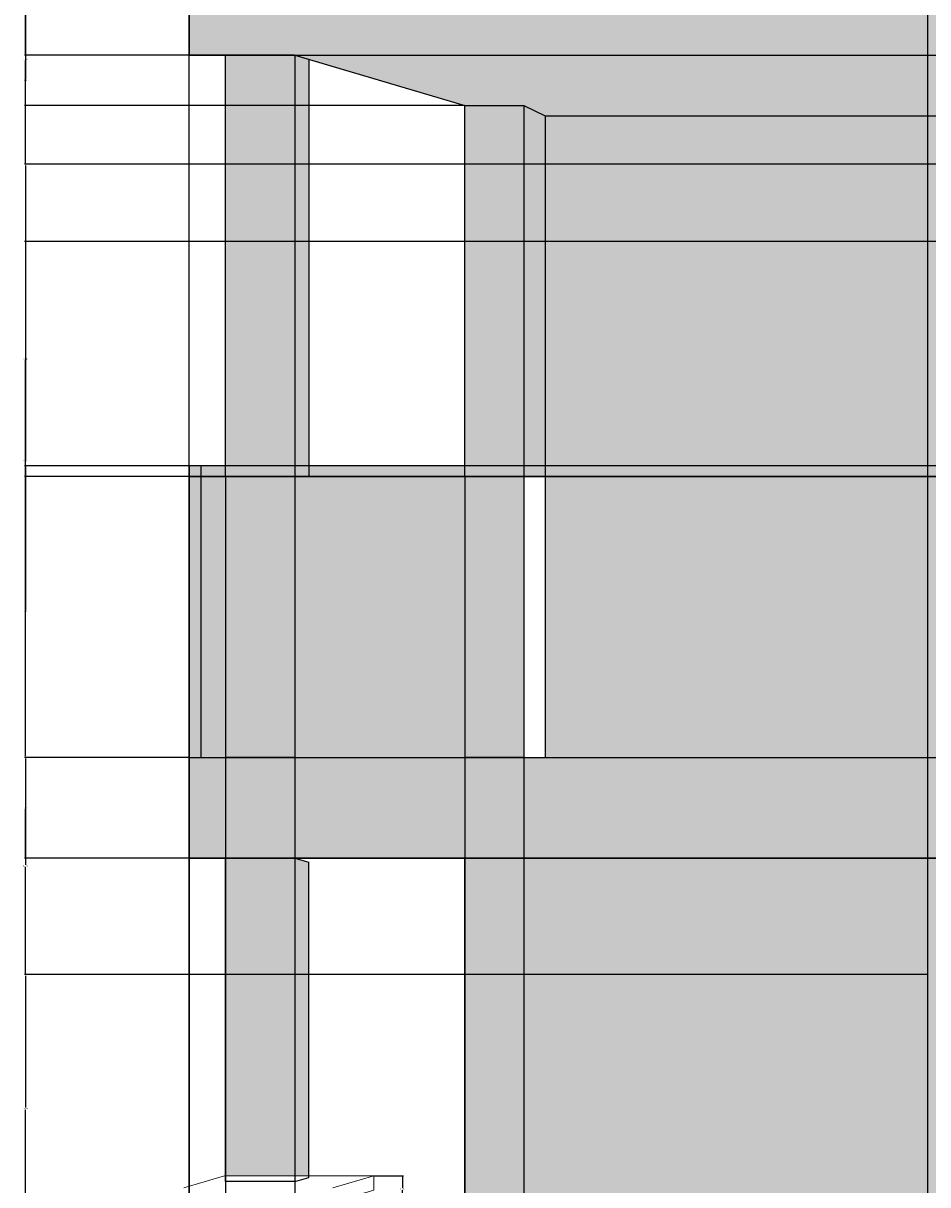
# Model space of a CAD drawing. Units: feet. Extents: x 2926 to 4178, y 965 to 1469.
# Tile 2 of 9: x 2926 to 3068, y 1059 to 1241. Entities that reach past the tile are written whole.
import ezdxf

# ---------------------------------------------------------------- set-up
doc = ezdxf.new("R2010")
doc.units = ezdxf.units.FT
for name, color, linetype, lineweight in [('A-ANNO-DIMS', 2, 'Continuous', 18), ('A-ELEV', 7, 'Continuous', 25), ('A-ELEV-DETL', 8, 'Continuous', 18), ('A-ELEV-PATT', 9, 'Continuous', 13)]:
    doc.layers.add(name, color=color, linetype=linetype, lineweight=lineweight)
doc.styles.get("Standard").update_dxf_attribs({"font": 'arial.ttf'})
doc.dimstyles.get("Standard").update_dxf_attribs({"dimtxt": 0.18, "dimasz": 0.18, "dimexe": 0.18, "dimexo": 0.0625, "dimgap": 0.09, "dimtad": 0, "dimtih": 1, "dimtoh": 1, "dimdec": 1, "dimzin": 0, "dimdsep": 46, "dimlunit": 3, "dimtxsty": 'Standard', "dimcen": 0.09, "dimadec": 0, "dimazin": 0, "dimtfac": 1, "dimtdec": 1, "dimtofl": 0, "dimtmove": 0, "dimatfit": 3, "dimfxl": 1, "dimtolj": 1, "dimtzin": 0, "dimarcsym": 0})

# ---------------------------------------------------------------- blocks, each defined once
blk = doc.blocks.new('PILLAR-CAP-A')
for p, q in [((0, 2.25), (6.42, 4.14)), ((0, 2.25), (6.42, 4.14)), ((29.85, 4.14), (6.42, 4.14)), ((29.85, 4.14), (6.42, 4.14)), ((23.43, 2.25), (29.85, 4.14)), ((23.43, 2.25), (29.85, 4.14)), ((29.85, 1.89), (29.85, 4.14)), ((29.85, 1.89), (29.85, 4.14)), ((23.43, 0), (29.85, 1.89)), ((23.43, 0), (29.85, 1.89))]:
    blk.add_line(p, q)
blk = doc.blocks.new('*D7')
at = {"layer": 'A-ANNO-DIMS', "color": 0, "lineweight": -2, "transparency": 16777216}
for p, q in [((2981.46, 1060.46), (2986.06, 1060.46)), ((2985.88, 1060.28), (2985.88, 1058.57)), ((2985.88, 1056.5), (2985.88, 1058.21)), ((2981.46, 1056.32), (2986.06, 1056.32))]:
    blk.add_line(p, q, dxfattribs=at)
at = {"layer": 'A-ANNO-DIMS', "color": 0, "transparency": 16777216}
for points in [[(2985.85, 1060.28), (2985.91, 1060.28), (2985.88, 1060.46)], [(2985.85, 1056.5), (2985.91, 1056.5), (2985.88, 1056.32)]]:
    blk.add_solid(points, dxfattribs=at)
at = {"layer": 'Defpoints', "color": 0, "transparency": 16777216}
for p in [(2981.4, 1060.46), (2985.88, 1060.46), (2981.4, 1056.32)]:
    blk.add_point(p, dxfattribs=at)
at = {"layer": 'A-ANNO-DIMS', "color": 0, "transparency": 16777216, "insert": (2985.88, 1058.39), "char_height": 0.18, "attachment_point": 5}
blk.add_mtext('\\A1;4 TYP.', dxfattribs=at)
blk = doc.blocks.new('*D14')
at = {"layer": 'A-ANNO-DIMS', "color": 0, "lineweight": -2, "transparency": 16777216}
for p, q in [((3068.25, 1092.04), (2926.57, 1092.04)), ((2926.75, 1091.86), (2926.75, 1071.2)), ((2926.75, 1050.16), (2926.75, 1070.83)), ((3068.25, 1049.98), (2926.57, 1049.98))]:
    blk.add_line(p, q, dxfattribs=at)
at = {"layer": 'A-ANNO-DIMS', "color": 0, "transparency": 16777216}
for points in [[(2926.72, 1091.86), (2926.78, 1091.86), (2926.75, 1092.04)], [(2926.72, 1050.16), (2926.78, 1050.16), (2926.75, 1049.98)]]:
    blk.add_solid(points, dxfattribs=at)
at = {"layer": 'Defpoints', "color": 0, "transparency": 16777216}
for p in [(2926.75, 1092.04), (3068.31, 1092.04), (3068.31, 1049.98)]:
    blk.add_point(p, dxfattribs=at)
at = {"layer": 'A-ANNO-DIMS', "color": 0, "transparency": 16777216, "insert": (2926.75, 1071.01), "char_height": 0.18, "attachment_point": 5}
blk.add_mtext('\\A1;42.06', dxfattribs=at)
blk = doc.blocks.new('*D15')
at = {"layer": 'A-ANNO-DIMS', "color": 0, "lineweight": -2, "transparency": 16777216}
for p, q in [((2952.34, 1126.14), (2926.57, 1126.14)), ((2926.75, 1125.96), (2926.75, 1109.27)), ((2926.75, 1092.22), (2926.75, 1108.91)), ((3068.25, 1092.04), (2926.57, 1092.04))]:
    blk.add_line(p, q, dxfattribs=at)
at = {"layer": 'A-ANNO-DIMS', "color": 0, "transparency": 16777216}
for points in [[(2926.72, 1125.96), (2926.78, 1125.96), (2926.75, 1126.14)], [(2926.72, 1092.22), (2926.78, 1092.22), (2926.75, 1092.04)]]:
    blk.add_solid(points, dxfattribs=at)
at = {"layer": 'Defpoints', "color": 0, "transparency": 16777216}
for p in [(2926.75, 1126.14), (2952.4, 1126.14), (3068.31, 1092.04)]:
    blk.add_point(p, dxfattribs=at)
at = {"layer": 'A-ANNO-DIMS', "color": 0, "transparency": 16777216, "insert": (2926.75, 1109.09), "char_height": 0.18, "attachment_point": 5}
blk.add_mtext('\\A1;34.095', dxfattribs=at)
blk = doc.blocks.new('*D16')
at = {"layer": 'A-ANNO-DIMS', "color": 0, "lineweight": -2, "transparency": 16777216}
for p, q in [((3198.58, 1219.22), (2926.57, 1219.22)), ((2926.75, 1219.04), (2926.75, 1172.86)), ((2926.75, 1126.32), (2926.75, 1172.5)), ((2952.34, 1126.14), (2926.57, 1126.14))]:
    blk.add_line(p, q, dxfattribs=at)
at = {"layer": 'A-ANNO-DIMS', "color": 0, "transparency": 16777216}
for points in [[(2926.72, 1219.04), (2926.78, 1219.04), (2926.75, 1219.22)], [(2926.72, 1126.32), (2926.78, 1126.32), (2926.75, 1126.14)]]:
    blk.add_solid(points, dxfattribs=at)
at = {"layer": 'Defpoints', "color": 0, "transparency": 16777216}
for p in [(2926.75, 1219.22), (3198.64, 1219.22), (2952.4, 1126.14)]:
    blk.add_point(p, dxfattribs=at)
at = {"layer": 'A-ANNO-DIMS', "color": 0, "transparency": 16777216, "insert": (2926.75, 1172.68), "char_height": 0.18, "attachment_point": 5}
blk.add_mtext('\\A1;93.08', dxfattribs=at)
blk = doc.blocks.new('*D17')
at = {"layer": 'A-ANNO-DIMS', "color": 0, "lineweight": -2, "transparency": 16777216}
for p, q in [((2952.34, 1252.14), (2926.57, 1252.14)), ((2926.75, 1251.96), (2926.75, 1235.86)), ((2926.75, 1219.4), (2926.75, 1235.5)), ((3198.58, 1219.22), (2926.57, 1219.22))]:
    blk.add_line(p, q, dxfattribs=at)
at = {"layer": 'A-ANNO-DIMS', "color": 0, "transparency": 16777216}
for points in [[(2926.72, 1251.96), (2926.78, 1251.96), (2926.75, 1252.14)], [(2926.72, 1219.4), (2926.78, 1219.4), (2926.75, 1219.22)]]:
    blk.add_solid(points, dxfattribs=at)
at = {"layer": 'Defpoints', "color": 0, "transparency": 16777216}
for p in [(2926.75, 1252.14), (2952.4, 1252.14), (3198.64, 1219.22)]:
    blk.add_point(p, dxfattribs=at)
at = {"layer": 'A-ANNO-DIMS', "color": 0, "transparency": 16777216, "insert": (2926.75, 1235.68), "char_height": 0.18, "attachment_point": 5}
blk.add_mtext('\\A1;32.92', dxfattribs=at)
blk = doc.blocks.new('*D22')
at = {"layer": 'A-ANNO-DIMS', "color": 0, "lineweight": -2, "transparency": 16777216}
for p, q in [((2952.4, 1056.38), (2952.4, 1468.62)), ((2952.58, 1468.44), (3009.97, 1468.44)), ((3068.13, 1468.44), (3010.74, 1468.44)), ((3068.31, 1050.05), (3068.31, 1468.62))]:
    blk.add_line(p, q, dxfattribs=at)
at = {"layer": 'A-ANNO-DIMS', "color": 0, "transparency": 16777216}
for points in [[(2952.58, 1468.47), (2952.58, 1468.41), (2952.4, 1468.44)], [(3068.13, 1468.47), (3068.13, 1468.41), (3068.31, 1468.44)]]:
    blk.add_solid(points, dxfattribs=at)
at = {"layer": 'Defpoints', "color": 0, "transparency": 16777216}
for p in [(3068.31, 1468.44), (2952.4, 1056.32), (3068.31, 1049.98)]:
    blk.add_point(p, dxfattribs=at)
at = {"layer": 'A-ANNO-DIMS', "color": 0, "transparency": 16777216, "insert": (3010.36, 1468.44), "char_height": 0.18, "attachment_point": 5}
blk.add_mtext('\\A1;115.9', dxfattribs=at)
blk = doc.blocks.new('*D23')
at = {"layer": 'A-ANNO-DIMS', "color": 0, "lineweight": -2, "transparency": 16777216}
for p, q in [((3068.31, 1050.05), (3068.31, 1468.62)), ((3068.49, 1468.44), (3099.11, 1468.44)), ((3130.51, 1468.44), (3099.9, 1468.44)), ((3130.69, 1050.05), (3130.69, 1468.62))]:
    blk.add_line(p, q, dxfattribs=at)
at = {"layer": 'A-ANNO-DIMS', "color": 0, "transparency": 16777216}
for points in [[(3068.49, 1468.47), (3068.49, 1468.41), (3068.31, 1468.44)], [(3130.51, 1468.47), (3130.51, 1468.41), (3130.69, 1468.44)]]:
    blk.add_solid(points, dxfattribs=at)
at = {"layer": 'Defpoints', "color": 0, "transparency": 16777216}
for p in [(3130.69, 1468.44), (3068.31, 1049.98), (3130.69, 1049.98)]:
    blk.add_point(p, dxfattribs=at)
at = {"layer": 'A-ANNO-DIMS', "color": 0, "transparency": 16777216, "insert": (3099.5, 1468.44), "char_height": 0.18, "attachment_point": 5}
blk.add_mtext('\\A1;62.38', dxfattribs=at)
blk = doc.blocks.new('*D50')
at = {"layer": 'A-ANNO-DIMS', "color": 0, "lineweight": -2, "transparency": 16777216}
for p, q in [((2952.4, 1171.83), (2952.4, 965.34)), ((2958.11, 1170.16), (2958.11, 965.34)), ((2952.58, 965.52), (2954.87, 965.52)), ((2957.93, 965.52), (2955.65, 965.52))]:
    blk.add_line(p, q, dxfattribs=at)
at = {"layer": 'A-ANNO-DIMS', "color": 0, "transparency": 16777216}
for points in [[(2952.58, 965.55), (2952.58, 965.49), (2952.4, 965.52)], [(2957.93, 965.55), (2957.93, 965.49), (2958.11, 965.52)]]:
    blk.add_solid(points, dxfattribs=at)
at = {"layer": 'Defpoints', "color": 0, "transparency": 16777216}
for p in [(2952.4, 1171.9), (2958.11, 1170.22), (2958.11, 965.52)]:
    blk.add_point(p, dxfattribs=at)
at = {"layer": 'A-ANNO-DIMS', "color": 0, "transparency": 16777216, "insert": (2955.26, 965.52), "char_height": 0.18, "attachment_point": 5}
blk.add_mtext('\\A1;5.712', dxfattribs=at)
blk = doc.blocks.new('*D51')
at = {"layer": 'A-ANNO-DIMS', "color": 0, "lineweight": -2, "transparency": 16777216}
for p, q in [((2958.11, 1170.16), (2958.11, 965.34)), ((2968.99, 1170.16), (2968.99, 965.34)), ((2958.29, 965.52), (2963.11, 965.52)), ((2968.81, 965.52), (2963.99, 965.52))]:
    blk.add_line(p, q, dxfattribs=at)
at = {"layer": 'A-ANNO-DIMS', "color": 0, "transparency": 16777216}
for points in [[(2958.29, 965.55), (2958.29, 965.49), (2958.11, 965.52)], [(2968.81, 965.55), (2968.81, 965.49), (2968.99, 965.52)]]:
    blk.add_solid(points, dxfattribs=at)
at = {"layer": 'Defpoints', "color": 0, "transparency": 16777216}
for p in [(2958.11, 1170.22), (2968.99, 1170.22), (2968.99, 965.52)]:
    blk.add_point(p, dxfattribs=at)
at = {"layer": 'A-ANNO-DIMS', "color": 0, "transparency": 16777216, "insert": (2963.55, 965.52), "char_height": 0.18, "attachment_point": 5}
blk.add_mtext('\\A1;10.871', dxfattribs=at)
blk = doc.blocks.new('*D52')
at = {"layer": 'A-ANNO-DIMS', "color": 0, "lineweight": -2, "transparency": 16777216}
for p, q in [((2968.99, 1170.16), (2968.99, 965.34)), ((2995.67, 1170.16), (2995.67, 965.34)), ((2969.17, 965.52), (2981.86, 965.52)), ((2995.49, 965.52), (2982.79, 965.52))]:
    blk.add_line(p, q, dxfattribs=at)
at = {"layer": 'A-ANNO-DIMS', "color": 0, "transparency": 16777216}
for points in [[(2969.17, 965.55), (2969.17, 965.49), (2968.99, 965.52)], [(2995.49, 965.55), (2995.49, 965.49), (2995.67, 965.52)]]:
    blk.add_solid(points, dxfattribs=at)
at = {"layer": 'Defpoints', "color": 0, "transparency": 16777216}
for p in [(2968.99, 1170.22), (2995.67, 1170.22), (2995.67, 965.52)]:
    blk.add_point(p, dxfattribs=at)
at = {"layer": 'A-ANNO-DIMS', "color": 0, "transparency": 16777216, "insert": (2982.33, 965.52), "char_height": 0.18, "attachment_point": 5}
blk.add_mtext('\\A1;26.685', dxfattribs=at)
blk = doc.blocks.new('*D53')
at = {"layer": 'A-ANNO-DIMS', "color": 0, "lineweight": -2, "transparency": 16777216}
for p, q in [((3004.93, 1228.4), (3004.93, 965.34)), ((2995.67, 1170.16), (2995.67, 965.34)), ((2995.85, 965.52), (2999.91, 965.52)), ((3004.75, 965.52), (3000.69, 965.52))]:
    blk.add_line(p, q, dxfattribs=at)
at = {"layer": 'A-ANNO-DIMS', "color": 0, "transparency": 16777216}
for points in [[(2995.85, 965.55), (2995.85, 965.49), (2995.67, 965.52)], [(3004.75, 965.55), (3004.75, 965.49), (3004.93, 965.52)]]:
    blk.add_solid(points, dxfattribs=at)
at = {"layer": 'Defpoints', "color": 0, "transparency": 16777216}
for p in [(3004.93, 1228.46), (2995.67, 1170.22), (3004.93, 965.52)]:
    blk.add_point(p, dxfattribs=at)
at = {"layer": 'A-ANNO-DIMS', "color": 0, "transparency": 16777216, "insert": (3000.3, 965.52), "char_height": 0.18, "attachment_point": 5}
blk.add_mtext('\\A1;9.257', dxfattribs=at)
blk = doc.blocks.new('*D54')
at = {"layer": 'A-ANNO-DIMS', "color": 0, "lineweight": -2, "transparency": 16777216}
for p, q in [((3004.93, 1228.4), (3004.93, 965.34)), ((3084.03, 1170.16), (3084.03, 965.34)), ((3005.11, 965.52), (3044.17, 965.52)), ((3083.85, 965.52), (3044.79, 965.52))]:
    blk.add_line(p, q, dxfattribs=at)
at = {"layer": 'A-ANNO-DIMS', "color": 0, "transparency": 16777216}
for points in [[(3005.11, 965.55), (3005.11, 965.49), (3004.93, 965.52)], [(3083.85, 965.55), (3083.85, 965.49), (3084.03, 965.52)]]:
    blk.add_solid(points, dxfattribs=at)
at = {"layer": 'Defpoints', "color": 0, "transparency": 16777216}
for p in [(3004.93, 1228.46), (3084.03, 1170.22), (3084.03, 965.52)]:
    blk.add_point(p, dxfattribs=at)
at = {"layer": 'A-ANNO-DIMS', "color": 0, "transparency": 16777216, "insert": (3044.48, 965.52), "char_height": 0.18, "attachment_point": 5}
blk.add_mtext('\\A1;79.1', dxfattribs=at)
blk = doc.blocks.new('*D57')
at = {"layer": 'A-ANNO-DIMS', "color": 0, "lineweight": -2, "transparency": 16777216}
for p, q in [((3154.71, 1207.11), (2926.57, 1207.11)), ((2926.75, 1206.93), (2926.75, 1188.84)), ((2926.75, 1170.4), (2926.75, 1188.48)), ((3154.71, 1170.22), (2926.57, 1170.22))]:
    blk.add_line(p, q, dxfattribs=at)
at = {"layer": 'A-ANNO-DIMS', "color": 0, "transparency": 16777216}
for points in [[(2926.72, 1206.93), (2926.78, 1206.93), (2926.75, 1207.11)], [(2926.72, 1170.4), (2926.78, 1170.4), (2926.75, 1170.22)]]:
    blk.add_solid(points, dxfattribs=at)
at = {"layer": 'Defpoints', "color": 0, "transparency": 16777216}
for p in [(2926.75, 1207.11), (3154.77, 1207.11), (3154.77, 1170.22)]:
    blk.add_point(p, dxfattribs=at)
at = {"layer": 'A-ANNO-DIMS', "color": 0, "transparency": 16777216, "insert": (2926.75, 1188.66), "char_height": 0.18, "attachment_point": 5}
blk.add_mtext('\\A1;36.89', dxfattribs=at)
blk = doc.blocks.new('*D58')
at = {"layer": 'A-ANNO-DIMS', "color": 0, "lineweight": -2, "transparency": 16777216}
for p, q in [((2968.92, 1236.32), (2926.57, 1236.32)), ((2926.75, 1236.14), (2926.75, 1232.58)), ((2926.75, 1228.64), (2926.75, 1232.21)), ((2995.61, 1228.46), (2926.57, 1228.46))]:
    blk.add_line(p, q, dxfattribs=at)
at = {"layer": 'A-ANNO-DIMS', "color": 0, "transparency": 16777216}
for points in [[(2926.72, 1236.14), (2926.78, 1236.14), (2926.75, 1236.32)], [(2926.72, 1228.64), (2926.78, 1228.64), (2926.75, 1228.46)]]:
    blk.add_solid(points, dxfattribs=at)
at = {"layer": 'Defpoints', "color": 0, "transparency": 16777216}
for p in [(2926.75, 1236.32), (2968.99, 1236.32), (2995.67, 1228.46)]:
    blk.add_point(p, dxfattribs=at)
at = {"layer": 'A-ANNO-DIMS', "color": 0, "transparency": 16777216, "insert": (2926.75, 1232.39), "char_height": 0.18, "attachment_point": 5}
blk.add_mtext('\\A1;7.86', dxfattribs=at)
blk = doc.blocks.new('*D59')
at = {"layer": 'A-ANNO-DIMS', "color": 0, "lineweight": -2, "transparency": 16777216}
for p, q in [((2952.34, 1171.9), (2926.57, 1171.9)), ((2926.75, 1171.72), (2926.75, 1149.2)), ((2926.75, 1126.32), (2926.75, 1148.84)), ((2952.34, 1126.14), (2926.57, 1126.14))]:
    blk.add_line(p, q, dxfattribs=at)
at = {"layer": 'A-ANNO-DIMS', "color": 0, "transparency": 16777216}
for points in [[(2926.72, 1171.72), (2926.78, 1171.72), (2926.75, 1171.9)], [(2926.72, 1126.32), (2926.78, 1126.32), (2926.75, 1126.14)]]:
    blk.add_solid(points, dxfattribs=at)
at = {"layer": 'Defpoints', "color": 0, "transparency": 16777216}
for p in [(2926.75, 1171.9), (2952.4, 1171.9), (2952.4, 1126.14)]:
    blk.add_point(p, dxfattribs=at)
at = {"layer": 'A-ANNO-DIMS', "color": 0, "transparency": 16777216, "insert": (2926.75, 1149.02), "char_height": 0.18, "attachment_point": 5}
blk.add_mtext('\\A1;45.76', dxfattribs=at)
blk = doc.blocks.new('*D60')
at = {"layer": 'A-ANNO-DIMS', "color": 0, "lineweight": -2, "transparency": 16777216}
for p, q in [((2952.34, 1126.14), (2926.57, 1126.14)), ((2926.75, 1125.96), (2926.75, 1118.41)), ((2926.75, 1110.5), (2926.75, 1118.05)), ((2952.34, 1110.32), (2926.57, 1110.32))]:
    blk.add_line(p, q, dxfattribs=at)
at = {"layer": 'A-ANNO-DIMS', "color": 0, "transparency": 16777216}
for points in [[(2926.72, 1125.96), (2926.78, 1125.96), (2926.75, 1126.14)], [(2926.72, 1110.5), (2926.78, 1110.5), (2926.75, 1110.32)]]:
    blk.add_solid(points, dxfattribs=at)
at = {"layer": 'Defpoints', "color": 0, "transparency": 16777216}
for p in [(2926.75, 1126.14), (2952.4, 1126.14), (2952.4, 1110.32)]:
    blk.add_point(p, dxfattribs=at)
at = {"layer": 'A-ANNO-DIMS', "color": 0, "transparency": 16777216, "insert": (2926.75, 1118.23), "char_height": 0.18, "attachment_point": 5}
blk.add_mtext('\\A1;15.814', dxfattribs=at)
blk = doc.blocks.new('*D61')
at = {"layer": 'A-ANNO-DIMS', "color": 0, "lineweight": -2, "transparency": 16777216}
for p, q in [((2952.34, 1252.14), (2926.57, 1252.14)), ((2926.75, 1251.96), (2926.75, 1244.41)), ((2926.75, 1236.5), (2926.75, 1244.05)), ((2952.34, 1236.32), (2926.57, 1236.32))]:
    blk.add_line(p, q, dxfattribs=at)
at = {"layer": 'A-ANNO-DIMS', "color": 0, "transparency": 16777216}
for points in [[(2926.72, 1251.96), (2926.78, 1251.96), (2926.75, 1252.14)], [(2926.72, 1236.5), (2926.78, 1236.5), (2926.75, 1236.32)]]:
    blk.add_solid(points, dxfattribs=at)
at = {"layer": 'Defpoints', "color": 0, "transparency": 16777216}
for p in [(2926.75, 1252.14), (2952.4, 1252.14), (2952.4, 1236.32)]:
    blk.add_point(p, dxfattribs=at)
at = {"layer": 'A-ANNO-DIMS', "color": 0, "transparency": 16777216, "insert": (2926.75, 1244.23), "char_height": 0.18, "attachment_point": 5}
blk.add_mtext('\\A1;15.814', dxfattribs=at)

msp = doc.modelspace()

# ---------------------------------------------------------------- hatches: boundary and pattern name
at = {"layer": 'A-ELEV-PATT'}
h = msp.add_hatch(color=256, dxfattribs=at)
h.dxf.hatch_style = 1
h.paths.add_polyline_path([(2968.9852, 1110.3246), (2958.1139, 1110.3246), (2958.1139, 1060.462), (2968.9852, 1060.462)])
h.paths.add_polyline_path([(3174.217, 1126.1389), (2952.4018, 1126.1389), (2952.4018, 1110.3246), (3174.217, 1110.3246), (3273.5987, 1110.3246), (3273.5987, 1116.3246), (3174.217, 1116.3246)], flags=17)
h.paths.add_polyline_path([(3289.413, 1252.1389), (2952.4018, 1252.1389), (2952.4018, 1236.3246), (3273.5987, 1236.3246), (3273.5987, 1110.3246), (3289.413, 1110.3246)])
h.paths.add_polyline_path([(3221.3497, 1355.2778), (3042.9199, 1355.2778), (3042.9199, 1339.4635), (3221.3497, 1339.4635)])
h.paths.add_polyline_path([(3379.9311, 1355.2778), (3262.1646, 1355.2778), (3262.1646, 1339.4635), (3364.1168, 1339.4635), (3364.1168, 990.3246), (3379.9311, 990.3246)])
h.paths.add_polyline_path([(3364.1168, 1330.7444), (3335.9143, 1330.7444), (3335.9143, 1023.8561), (3364.1168, 1023.8561), (3364.1168, 1027.6935), (3339.7517, 1027.6935), (3339.7517, 1326.907), (3364.1168, 1326.907)], flags=17)
h.paths.add_polyline_path([(3438.5707, 1443.6445), (3153.6951, 1443.6445), (3153.6951, 1427.8302), (3438.5707, 1427.8302)])
h.paths.add_polyline_path([(3174.217, 1427.8302), (3153.6951, 1427.8302), (3174.217, 1356.4366)])
h.paths.add_polyline_path([(3174.217, 1339.4635), (3042.9199, 1339.4635), (3070.6809, 1317.1829), (3174.217, 1317.1829)])
h.paths.add_polyline_path([(3244.819, 1219.2195), (3198.6415, 1219.2195), (3198.6415, 1133.2879), (3244.819, 1133.2879)], flags=17)
h = msp.add_hatch(color=256, dxfattribs=at)
h.dxf.hatch_style = 1
h.paths.add_polyline_path([(3006.649, 1296.2176), (2952.4018, 1296.2176), (2952.4018, 1252.1389), (3006.649, 1252.1389)])
h.paths.add_polyline_path([(3084.0314, 1226.8042), (3008.2802, 1226.8042), (3008.2802, 1171.8963), (3084.0314, 1171.8963)])
h.paths.add_polyline_path([(3004.9276, 1228.4641), (2995.6704, 1228.4641), (2995.6704, 1171.8963), (3004.9276, 1171.8963)])
h.paths.add_polyline_path([(3174.217, 1236.3246), (3084.0314, 1236.3246), (3084.0314, 1171.8963), (3124.7575, 1171.8963), (3124.7575, 1207.1083), (3154.7729, 1207.1083), (3154.7729, 1171.8963), (3174.217, 1171.8963)])
h.paths.add_polyline_path([(3273.5987, 1236.3246), (3174.217, 1236.3246), (3174.217, 1171.8963), (3174.217, 1126.1389), (3174.217, 1116.3246), (3273.5987, 1116.3246)], flags=16)
h.paths.add_polyline_path([(3198.6415, 1219.2195), (3244.819, 1219.2195), (3244.819, 1133.2879), (3198.6415, 1133.2879)], flags=0)
h.paths.add_polyline_path([(3432.4018, 1427.8302), (3174.217, 1427.8302), (3174.217, 1356.4366), (3174.5501, 1355.2778), (3221.3497, 1355.2778), (3221.3497, 1364.3965), (3232.8063, 1364.3965), (3232.8063, 1355.2778), (3236.4098, 1355.2778), (3236.4098, 1364.3965), (3247.8663, 1364.3965), (3247.8663, 1355.2778), (3250.7081, 1355.2778), (3250.7081, 1364.3965), (3262.1646, 1364.3965), (3262.1646, 1355.2778), (3379.9311, 1355.2778), (3379.9311, 990.3246), (3432.4018, 990.3246)])
h.paths.add_polyline_path([(3068.3128, 1092.0439), (3130.6886, 1092.0439), (3130.6886, 1049.9841), (3146.6469, 1049.9841), (3146.6469, 1057.7915), (3145.2184, 1058.2122), (3145.2184, 1060.462), (3168.644, 1060.462), (3174.217, 1058.8204), (3174.217, 1110.3246), (3004.9276, 1110.3246), (3004.9276, 1049.9841), (3068.3128, 1049.9841)])
h.paths.add_polyline_path([(3174.217, 1056.3197), (3152.4954, 1056.3197), (3152.4954, 990.3246), (3174.217, 990.3246)])
h.paths.add_polyline_path([(2974.1234, 1056.3197), (2952.4018, 1056.3197), (2952.4018, 990.3246), (2974.1234, 990.3246)])
h.paths.add_polyline_path([(3004.9276, 1110.3246), (2995.6704, 1110.3246), (2995.6704, 1049.9841), (3004.9276, 1049.9841)])
h = msp.add_hatch(color=256, dxfattribs=at)
h.dxf.hatch_style = 1
h.paths.add_polyline_path([(3174.217, 1297.8963), (3172.3488, 1297.8963), (3006.649, 1297.8963), (3006.649, 1296.2176), (3087.9974, 1296.2176), (3087.9974, 1252.1389), (3089.8656, 1252.1389), (3089.8656, 1296.2176), (3172.3488, 1296.2176), (3172.3488, 1252.1389), (3174.217, 1252.1389)])
h.paths.add_polyline_path([(3102.4583, 1170.2176), (3172.3488, 1170.2176), (3172.3488, 1126.1389), (3174.217, 1126.1389), (3174.217, 1171.8963), (3172.3488, 1171.8963), (2952.4018, 1171.8963), (2952.4018, 1170.2176), (2952.4018, 1126.1389), (2954.27, 1126.1389), (2954.27, 1170.2176), (3100.5901, 1170.2176), (3100.5901, 1126.1389), (3102.4583, 1126.1389)])
h.paths.add_polyline_path([(3130.6886, 1092.0439), (3068.3128, 1092.0439), (3068.3128, 1049.9841), (3130.6886, 1049.9841)])
h.paths.add_polyline_path([(3099.0016, 1090.4638), (3099.0016, 1051.5643), (3069.893, 1051.5643), (3069.893, 1090.4638)], flags=16)
h.paths.add_polyline_path([(3099.9998, 1090.4638), (3129.1085, 1090.4638), (3129.1085, 1051.5643), (3099.9998, 1051.5643)], flags=16)
h.paths.add_polyline_path([(3067.2712, 1049.9841), (3060.102, 1049.9841), (3060.102, 990.3246), (3067.2712, 990.3246)])
h.paths.add_polyline_path([(3339.7517, 1326.907), (3364.1168, 1326.907), (3364.1168, 1330.7444), (3335.9143, 1330.7444), (3335.9143, 1023.8561), (3364.1168, 1023.8561), (3364.1168, 1027.6935), (3339.7517, 1027.6935)])
h.paths.add_polyline_path([(3154.7729, 1207.1083), (3124.7575, 1207.1083), (3124.7575, 1171.8963), (3126.8684, 1171.8963), (3126.8684, 1204.9974), (3152.6619, 1204.9974), (3152.6619, 1171.8963), (3154.7729, 1171.8963)])
h = msp.add_hatch(color=256, dxfattribs=at)
h.dxf.hatch_style = 1
h.paths.add_polyline_path([(3070.6809, 1296.2176), (3006.649, 1296.2176), (3006.649, 1252.1389), (3070.6809, 1252.1389)])
h.paths.add_polyline_path([(3087.9974, 1296.2176), (3070.6809, 1296.2176), (3070.6809, 1252.1389), (3087.9974, 1252.1389)])
h.paths.add_polyline_path([(3172.3488, 1296.2176), (3089.8656, 1296.2176), (3089.8656, 1252.1389), (3172.3488, 1252.1389)])
h.paths.add_polyline_path([(3152.6619, 1170.2176), (3126.8684, 1170.2176), (3126.8684, 1128.2498), (3152.6619, 1128.2498)], flags=17)
h.paths.add_polyline_path([(3152.6619, 1204.9974), (3126.8684, 1204.9974), (3126.8684, 1171.8963), (3152.6619, 1171.8963)])
h.paths.add_polyline_path([(3172.3488, 1170.2176), (3154.7729, 1170.2176), (3154.7729, 1126.1389), (3172.3488, 1126.1389)])
h.paths.add_polyline_path([(3154.7729, 1170.2176), (3152.6619, 1170.2176), (3152.6619, 1128.2498), (3126.8684, 1128.2498), (3126.8684, 1170.2176), (3124.7575, 1170.2176), (3124.7575, 1126.1389), (3154.7729, 1126.1389)])
h.paths.add_polyline_path([(3124.7575, 1170.2176), (3102.4583, 1170.2176), (3102.4583, 1126.1389), (3124.7575, 1126.1389)])
h.paths.add_polyline_path([(3100.5901, 1170.2176), (3084.0314, 1170.2176), (3084.0314, 1126.1389), (3100.5901, 1126.1389)])
h.paths.add_polyline_path([(3084.0314, 1170.2176), (3008.2802, 1170.2176), (3008.2802, 1126.1389), (3084.0314, 1126.1389)])
h.paths.add_polyline_path([(2995.6704, 1170.2176), (2971.1978, 1170.2176), (2971.1978, 1126.1389), (2995.6704, 1126.1389)])
h.paths.add_polyline_path([(3004.9276, 1170.2176), (2995.6704, 1170.2176), (2995.6704, 1126.1389), (3004.9276, 1126.1389)])
h.paths.add_polyline_path([(3364.1168, 1326.907), (3339.7517, 1326.907), (3339.7517, 1027.6935), (3364.1168, 1027.6935)])
h.paths.add_polyline_path([(3099.0016, 1090.4638), (3069.893, 1090.4638), (3069.893, 1051.5643), (3099.0016, 1051.5643)])
h.paths.add_polyline_path([(3129.1085, 1090.4638), (3099.9998, 1090.4638), (3099.9998, 1051.5643), (3129.1085, 1051.5643)])
h.paths.add_polyline_path([(2968.9852, 1170.2176), (2958.1139, 1170.2176), (2958.1139, 1126.1389), (2968.9852, 1126.1389)])
h.paths.add_polyline_path([(2958.1139, 1170.2176), (2954.27, 1170.2176), (2954.27, 1126.1389), (2958.1139, 1126.1389)])
h.paths.add_polyline_path([(2971.1978, 1170.2176), (2968.9852, 1170.2176), (2968.9852, 1126.1389), (2971.1978, 1126.1389)])
h = msp.add_hatch(color=256, dxfattribs=at)
h.dxf.hatch_style = 1
h.paths.add_polyline_path([(2968.9852, 1236.3246), (2958.1139, 1236.3246), (2958.1139, 1171.8963), (2968.9852, 1171.8963)])
h = msp.add_hatch(color=256, dxfattribs=at)
h.dxf.hatch_style = 1
h.paths.add_polyline_path([(2971.1978, 1235.6728), (2968.9852, 1236.3246), (2968.9852, 1171.8963), (2971.1978, 1171.8963)])
h.paths.add_polyline_path([(2971.1978, 1109.6728), (2968.9852, 1110.3246), (2968.9852, 1060.462), (2971.1978, 1060.462)])
h.paths.add_polyline_path([(3084.0314, 1236.3246), (2968.9852, 1236.3246), (2995.6704, 1228.4641), (3004.9276, 1228.4641), (3008.2802, 1226.8042), (3084.0314, 1226.8042)])
h = msp.add_hatch(color=256, dxfattribs=at)
h.dxf.hatch_style = 1
h.paths.add_polyline_path([(2980.5295, 1057.9557), (2974.9754, 1056.3197), (2974.1234, 1056.3197), (2974.1234, 990.3246), (2977.7283, 990.3246), (2977.7283, 1049.9841), (2980.5295, 1049.9841)])
h.paths.add_polyline_path([(3152.4954, 1056.3197), (3151.6434, 1056.3197), (3146.6469, 1057.7915), (3146.6469, 1049.9841), (3149.6449, 1049.9841), (3149.6449, 990.3246), (3152.4954, 990.3246)])
h.paths.add_polyline_path([(3008.2802, 1226.8042), (3004.9276, 1228.4641), (3004.9276, 1171.8963), (3008.2802, 1171.8963)])

# ---------------------------------------------------------------- linework, layer by layer
at = {"layer": 'A-ELEV'}
for p, q in [((2952.4018, 1236.3246), (2952.4018, 1298.3338)), ((2952.4018, 1236.3246), (2952.4018, 1298.3338)), ((2952.4018, 1236.3246), (3273.5987, 1236.3246)), ((2952.4018, 1236.3246), (3273.5987, 1236.3246)), ((2968.9852, 1236.3246), (2995.6704, 1228.4641)), ((2968.9852, 1236.3246), (2995.6704, 1228.4641)), ((2971.1978, 1235.6728), (2971.1978, 1170.2176)), ((3004.9276, 1228.4641), (3008.2802, 1226.8042)), ((3004.9276, 1228.4641), (3008.2802, 1226.8042)), ((3008.2802, 1226.8042), (3008.2802, 1126.1389)), ((3008.2802, 1226.8042), (3084.0314, 1226.8042)), ((3008.2802, 1226.8042), (3008.2802, 1126.1389)), ((3008.2802, 1226.8042), (3084.0314, 1226.8042)), ((2952.4018, 1110.3246), (2952.4018, 1126.1389)), ((2952.4018, 1110.3246), (2952.4018, 1126.1389)), ((2952.4018, 1110.3246), (3289.413, 1110.3246)), ((2952.4018, 1110.3246), (3289.413, 1110.3246)), ((2968.9852, 1110.3246), (2971.1978, 1109.6728)), ((2968.9852, 1110.3246), (2971.1978, 1109.6728)), ((2971.1978, 1060.2025), (2971.1978, 1109.6728)), ((2971.1978, 1060.2025), (2971.1978, 1109.6728)), ((2968.9852, 1059.5508), (2971.1978, 1060.2025)), ((2968.9852, 1059.5508), (2971.1978, 1060.2025))]:
    msp.add_line(p, q, dxfattribs=at)
for points in [[(3289.413, 1236.3246), (3289.413, 1252.1389), (2952.4018, 1252.1389), (2952.4018, 1236.3246), (3273.5987, 1236.3246)], [(3289.413, 1236.3246), (3289.413, 1252.1389), (2952.4018, 1252.1389), (2952.4018, 1236.3246), (3273.5987, 1236.3246)], [(2958.1139, 1170.2176), (2958.1139, 1236.3246), (2968.9852, 1236.3246), (2968.9852, 1170.2176)], [(2995.6704, 1170.2176), (2995.6704, 1228.4641), (3004.9276, 1228.4641), (3004.9276, 1126.1389), (2995.6704, 1126.1389)], [(3174.217, 1110.3246), (2952.4018, 1110.3246), (2952.4018, 1126.1389), (3174.217, 1126.1389), (3174.217, 1116.3246)], [(3174.217, 1110.3246), (2952.4018, 1110.3246), (2952.4018, 1126.1389), (3174.217, 1126.1389), (3174.217, 1116.3246)], [(2968.9852, 1126.1389), (2958.1139, 1126.1389)]]:
    msp.add_lwpolyline(points, dxfattribs=at)
for points in [[(2952.4018, 1126.1389), (2954.27, 1126.1389), (2954.27, 1171.8963), (2952.4018, 1171.8963)], [(2952.4018, 1170.2176), (3174.217, 1170.2176), (3174.217, 1171.8963), (2952.4018, 1171.8963)], [(2952.4018, 1126.1389), (2954.27, 1126.1389), (2954.27, 1171.8963), (2952.4018, 1171.8963)], [(2952.4018, 1170.2176), (3174.217, 1170.2176), (3174.217, 1171.8963), (2952.4018, 1171.8963)], [(2958.1139, 1110.3246), (2968.9852, 1110.3246), (2968.9852, 1059.5508), (2958.1139, 1059.5508)], [(2958.1139, 1110.3246), (2968.9852, 1110.3246), (2968.9852, 1059.5508), (2958.1139, 1059.5508)], [(2995.6704, 1110.3246), (3004.9276, 1110.3246), (3004.9276, 1049.9841), (2995.6704, 1049.9841)], [(2995.6704, 1110.3246), (3004.9276, 1110.3246), (3004.9276, 1049.9841), (2995.6704, 1049.9841)]]:
    msp.add_lwpolyline(points, close=True, dxfattribs=at)

# ---------------------------------------------------------------- block references
at = {"layer": 'A-ELEV-DETL'}
msp.add_blockref('PILLAR-CAP-A', (2951.55, 1056.32), dxfattribs=at)

# ---------------------------------------------------------------- dimensions: what is measured, and where the dimension line sits
at = {"layer": 'A-ANNO-DIMS'}
for base, p1, p2, override, picture, middle in [((3068.3128, 1468.4445), (2952.4018, 1056.3197), (3068.3128, 1049.9841), {"dimdec": 1, "dimlfac": 1, "dimrnd": 0, "dimzin": 0, "dimdsep": 46, "dimlunit": 2}, '*D22', (3010.3573, 1468.4445)), ((3130.6886, 1468.4445), (3068.3128, 1049.9841), (3130.6886, 1049.9841), {"dimdec": 2, "dimlfac": 1, "dimrnd": 0, "dimzin": 0, "dimdsep": 46, "dimlunit": 2}, '*D23', (3099.5007, 1468.4445)), ((3004.9276, 965.5246), (2995.6704, 1170.2176), (3004.9276, 1228.4641), {"dimdec": 3, "dimlfac": 1, "dimrnd": 0, "dimzin": 0, "dimdsep": 46, "dimlunit": 2}, '*D53', (3000.299, 965.5246)), ((3084.0314, 965.5246), (3004.9276, 1228.4641), (3084.0314, 1170.2176), {"dimdec": 1, "dimlfac": 1, "dimrnd": 0, "dimzin": 0, "dimdsep": 46, "dimlunit": 2}, '*D54', (3044.4795, 965.5246)), ((2958.1139, 965.5246), (2952.4018, 1171.8963), (2958.1139, 1170.2176), {"dimdec": 3, "dimlfac": 1, "dimrnd": 0, "dimzin": 0, "dimdsep": 46, "dimlunit": 2}, '*D50', (2955.2579, 965.5246)), ((2968.9852, 965.5246), (2958.1139, 1170.2176), (2968.9852, 1170.2176), {"dimdec": 3, "dimlfac": 1, "dimrnd": 0, "dimzin": 0, "dimdsep": 46, "dimlunit": 2}, '*D51', (2963.5496, 965.5246)), ((2995.6704, 965.5246), (2968.9852, 1170.2176), (2995.6704, 1170.2176), {"dimdec": 3, "dimlfac": 1, "dimrnd": 0, "dimzin": 0, "dimdsep": 46, "dimlunit": 2}, '*D52', (2982.3278, 965.5246))]:
    dim = msp.add_linear_dim(base=base, p1=p1, p2=p2, dimstyle='Standard', override=override, dxfattribs=at)
    dim.commit()
    dim.dimension.update_dxf_attribs({"geometry": picture, "text_midpoint": middle})
for base, p1, p2, override, picture, middle in [((2926.7498, 1252.1389), (2952.4018, 1236.3246), (2952.4018, 1252.1389), {"dimdec": 3, "dimlfac": 1, "dimrnd": 0, "dimzin": 0, "dimdsep": 46, "dimlunit": 2}, '*D61', (2926.7498, 1244.2317)), ((2926.7498, 1252.1389), (3198.6415, 1219.2195), (2952.4018, 1252.1389), {"dimdec": 2, "dimlfac": 1, "dimrnd": 0, "dimzin": 0, "dimdsep": 46, "dimlunit": 2}, '*D17', (2926.7498, 1235.6792)), ((2926.7498, 1236.3246), (2995.6704, 1228.4641), (2968.9852, 1236.3246), {"dimdec": 2, "dimlfac": 1, "dimrnd": 0, "dimzin": 0, "dimdsep": 46, "dimlunit": 2}, '*D58', (2926.7498, 1232.3943)), ((2926.7498, 1219.2195), (2952.4018, 1126.1389), (3198.6415, 1219.2195), {"dimdec": 2, "dimlfac": 1, "dimrnd": 0, "dimzin": 0, "dimdsep": 46, "dimlunit": 2}, '*D16', (2926.7498, 1172.6792)), ((2926.7498, 1207.1083), (3154.7729, 1170.2176), (3154.7729, 1207.1083), {"dimdec": 2, "dimlfac": 1, "dimrnd": 0, "dimzin": 0, "dimdsep": 46, "dimlunit": 2}, '*D57', (2926.7498, 1188.663)), ((2926.7498, 1171.8963), (2952.4018, 1126.1389), (2952.4018, 1171.8963), {"dimdec": 2, "dimlfac": 1, "dimrnd": 0, "dimzin": 0, "dimdsep": 46, "dimlunit": 2}, '*D59', (2926.7498, 1149.0176)), ((2926.7498, 1126.1389), (3068.3128, 1092.0439), (2952.4018, 1126.1389), {"dimdec": 3, "dimlfac": 1, "dimrnd": 0, "dimzin": 0, "dimdsep": 46, "dimlunit": 2}, '*D15', (2926.7498, 1109.0914)), ((2926.7498, 1126.1389), (2952.4018, 1110.3246), (2952.4018, 1126.1389), {"dimdec": 3, "dimlfac": 1, "dimrnd": 0, "dimzin": 0, "dimdsep": 46, "dimlunit": 2}, '*D60', (2926.7498, 1118.2317)), ((2926.7498, 1092.0439), (3068.3128, 1049.9841), (3068.3128, 1092.0439), {"dimdec": 2, "dimlfac": 1, "dimrnd": 0, "dimzin": 0, "dimdsep": 46, "dimlunit": 2}, '*D14', (2926.7498, 1071.014))]:
    dim = msp.add_linear_dim(base=base, p1=p1, p2=p2, angle=90, dimstyle='Standard', override=override, dxfattribs=at)
    dim.commit()
    dim.dimension.update_dxf_attribs({"geometry": picture, "text_midpoint": middle})
dim = msp.add_linear_dim(base=(2985.878, 1060.462), p1=(2981.4004, 1056.3197), p2=(2981.4004, 1060.462), angle=90, text='<> TYP.', dimstyle='Standard', override={"dimdec": 0, "dimlfac": 1, "dimrnd": 0, "dimzin": 0, "dimdsep": 46, "dimlunit": 2}, dxfattribs=at)
dim.commit()
dim.dimension.update_dxf_attribs({"geometry": '*D7', "text_midpoint": (2985.878, 1058.3908)})

doc.saveas('drawing.dxf')
